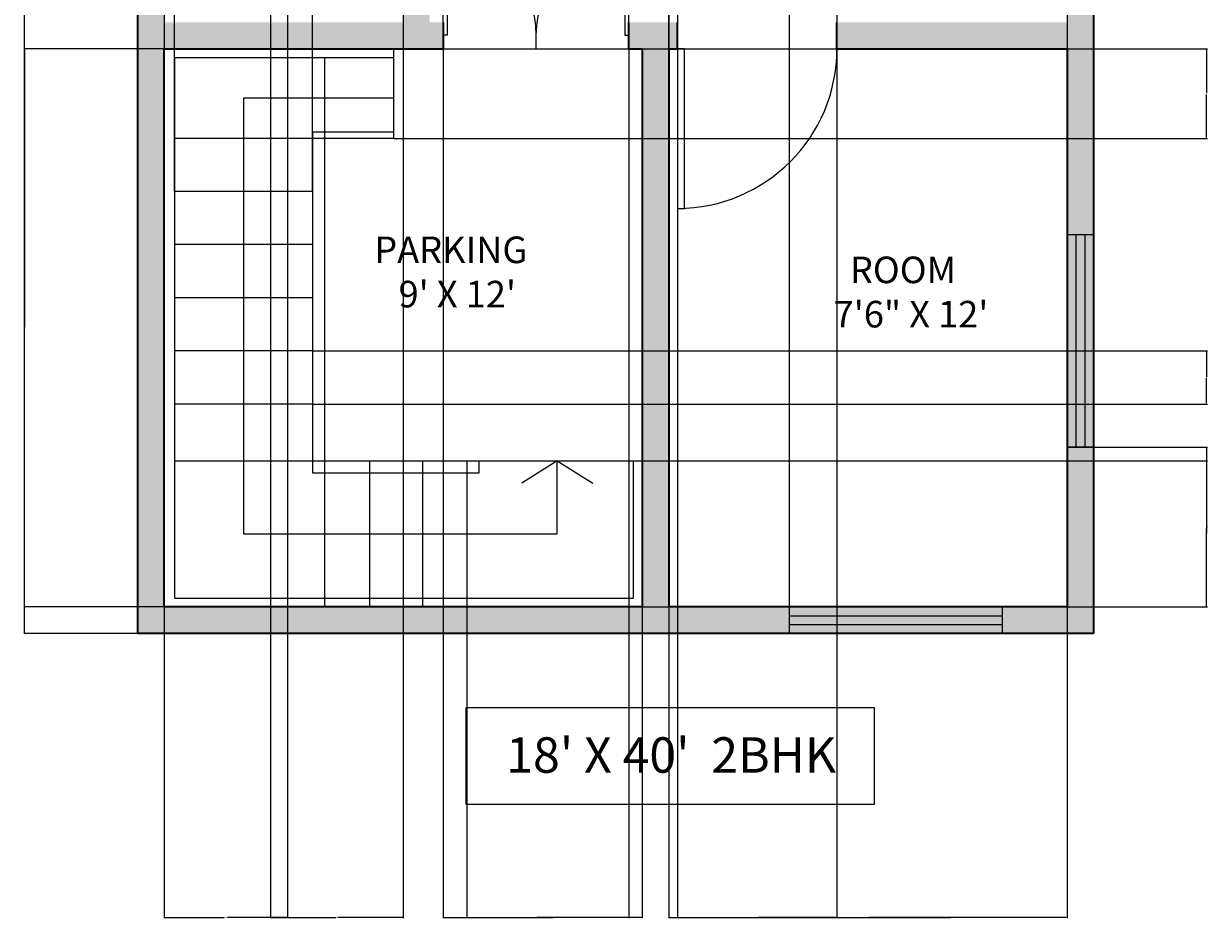
# Model space of a CAD drawing. Units: feet. Extents: x 4596233 to 4596501, y 5666486 to 5667044.
# Tile 1 of 3: x 4596233 to 4596501, y 5666486 to 5666688. Entities that reach past the tile are written whole.
import ezdxf

# ---------------------------------------------------------------- set-up
doc = ezdxf.new("R2010")
doc.units = ezdxf.units.FT
for name, color, linetype, lineweight in [('A-ANNO-DIMS', 2, 'Continuous', 18), ('A-ANNO-TTLB', 6, 'Continuous', 25), ('A-WALL', 7, 'Continuous', 35), ('ANNOTATION', 170, 'Continuous', 18), ('DOOR', 240, 'Continuous', 18), ('STAIR', 90, 'Continuous', 25)]:
    doc.layers.add(name, color=color, linetype=linetype, lineweight=lineweight)
doc.layers.add('A-GLAZ', color=2, linetype='Continuous', lineweight=18, true_color=0xf1eb1f)
doc.layers.add('A-WALL-PATT', color=251, linetype='Continuous', lineweight=13, true_color=0x636466)
doc.styles.get("Standard").update_dxf_attribs({"font": 'arial.ttf'})
doc.dimstyles.get("Standard").update_dxf_attribs({"dimtxt": 0.18, "dimasz": 0.18, "dimexe": 0.18, "dimexo": 0.0625, "dimgap": 0.09, "dimtad": 0, "dimtih": 1, "dimtoh": 1, "dimdec": 0, "dimzin": 0, "dimdsep": 46, "dimlunit": 3, "dimtxsty": 'Standard', "dimcen": 0.09, "dimadec": 0, "dimazin": 0, "dimtfac": 1, "dimtdec": 0, "dimtofl": 0, "dimtmove": 0, "dimatfit": 3, "dimfxl": 1, "dimtolj": 1, "dimtzin": 0, "dimarcsym": 0})

# ---------------------------------------------------------------- blocks, each defined once
blk = doc.blocks.new('*U3')
for p, q in [((0, 0), (0, -6)), ((-40, 0), (-40, -6))]:
    blk.add_line(p, q)
blk.add_lwpolyline([(0, 0), (0, 40), (-1.75, 40), (-1.75, 0)], close=True)
blk.add_arc((0, 0), 40, 90, 180)
blk = doc.blocks.new('*U4')
for p, q in [((0, 0), (0, 6)), ((40, 0), (40, 6))]:
    blk.add_line(p, q)
blk.add_lwpolyline([(0, 0), (0, -40), (1.75, -40), (1.75, 0)], close=True)
blk.add_arc((0, 0), 40, 270, 0)
blk = doc.blocks.new('WIN-48IN')
h = blk.add_hatch(color=256)
h.dxf.hatch_style = 1
h.paths.add_polyline_path([(48, 2), (48, 4), (0, 4), (0, 2)])
for p, q in [((0, 6), (48, 6)), ((0, 0), (0, 6)), ((48, 6), (48, 0)), ((0, 4), (48, 4)), ((0, 2), (48, 2)), ((48, 0), (0, 0))]:
    blk.add_line(p, q)
blk = doc.blocks.new('*D12')
at = {"layer": 'A-ANNO-DIMS', "color": 0, "lineweight": -2, "transparency": 16777216}
for p, q in [((4596258.79, 5667018.15), (4596233.12, 5667018.15)), ((4596233.3, 5667017.97), (4596233.3, 5666784.33)), ((4596233.3, 5666550.33), (4596233.3, 5666783.97)), ((4596258.79, 5666550.15), (4596233.12, 5666550.15))]:
    blk.add_line(p, q, dxfattribs=at)
at = {"layer": 'A-ANNO-DIMS', "color": 0, "transparency": 16777216}
for points in [[(4596233.27, 5667017.97), (4596233.33, 5667017.97), (4596233.3, 5667018.15)], [(4596233.27, 5666550.33), (4596233.33, 5666550.33), (4596233.3, 5666550.15)]]:
    blk.add_solid(points, dxfattribs=at)
at = {"layer": 'Defpoints', "color": 0, "transparency": 16777216}
for p in [(4596233.3, 5667018.15), (4596258.85, 5667018.15), (4596258.85, 5666550.15)]:
    blk.add_point(p, dxfattribs=at)
at = {"layer": 'A-ANNO-DIMS', "color": 0, "transparency": 16777216, "insert": (4596233.3, 5666784.15), "char_height": 0.18, "attachment_point": 5}
blk.add_mtext('\\A1;468', dxfattribs=at)
blk = doc.blocks.new('*D13')
at = {"layer": 'A-ANNO-DIMS', "color": 0, "lineweight": -2, "transparency": 16777216}
for p, q in [((4596264.79, 5666682.15), (4596233.12, 5666682.15)), ((4596233.3, 5666681.97), (4596233.3, 5666619.33)), ((4596233.3, 5666556.33), (4596233.3, 5666618.97)), ((4596264.79, 5666556.15), (4596233.12, 5666556.15))]:
    blk.add_line(p, q, dxfattribs=at)
at = {"layer": 'A-ANNO-DIMS', "color": 0, "transparency": 16777216}
for points in [[(4596233.27, 5666681.97), (4596233.33, 5666681.97), (4596233.3, 5666682.15)], [(4596233.27, 5666556.33), (4596233.33, 5666556.33), (4596233.3, 5666556.15)]]:
    blk.add_solid(points, dxfattribs=at)
at = {"layer": 'Defpoints', "color": 0, "transparency": 16777216}
for p in [(4596233.3, 5666682.15), (4596264.85, 5666682.15), (4596264.85, 5666556.15)]:
    blk.add_point(p, dxfattribs=at)
at = {"layer": 'A-ANNO-DIMS', "color": 0, "transparency": 16777216, "insert": (4596233.3, 5666619.15), "char_height": 0.18, "attachment_point": 5}
blk.add_mtext('\\A1;126', dxfattribs=at)
blk = doc.blocks.new('*D15')
at = {"layer": 'A-ANNO-DIMS', "color": 0, "lineweight": -2, "transparency": 16777216}
for p, q in [((4596378.85, 5666964.09), (4596378.85, 5666485.84)), ((4596468.85, 5666964.09), (4596468.85, 5666485.84)), ((4596379.03, 5666486.02), (4596423.63, 5666486.02)), ((4596468.67, 5666486.02), (4596424.07, 5666486.02))]:
    blk.add_line(p, q, dxfattribs=at)
at = {"layer": 'A-ANNO-DIMS', "color": 0, "transparency": 16777216}
for points in [[(4596379.03, 5666486.05), (4596379.03, 5666485.99), (4596378.85, 5666486.02)], [(4596468.67, 5666486.05), (4596468.67, 5666485.99), (4596468.85, 5666486.02)]]:
    blk.add_solid(points, dxfattribs=at)
at = {"layer": 'Defpoints', "color": 0, "transparency": 16777216}
for p in [(4596378.85, 5666964.15), (4596468.85, 5666964.15), (4596468.85, 5666486.02)]:
    blk.add_point(p, dxfattribs=at)
at = {"layer": 'A-ANNO-DIMS', "color": 0, "transparency": 16777216, "insert": (4596423.85, 5666486.02), "char_height": 0.18, "attachment_point": 5}
blk.add_mtext('\\A1;90', dxfattribs=at)
blk = doc.blocks.new('*D16')
at = {"layer": 'A-ANNO-DIMS', "color": 0, "lineweight": -2, "transparency": 16777216}
for p, q in [((4596327.85, 5666682.09), (4596327.85, 5666485.84)), ((4596369.85, 5666682.09), (4596369.85, 5666485.84)), ((4596328.03, 5666486.02), (4596348.63, 5666486.02)), ((4596369.67, 5666486.02), (4596349.07, 5666486.02))]:
    blk.add_line(p, q, dxfattribs=at)
at = {"layer": 'A-ANNO-DIMS', "color": 0, "transparency": 16777216}
for points in [[(4596328.03, 5666486.05), (4596328.03, 5666485.99), (4596327.85, 5666486.02)], [(4596369.67, 5666486.05), (4596369.67, 5666485.99), (4596369.85, 5666486.02)]]:
    blk.add_solid(points, dxfattribs=at)
at = {"layer": 'Defpoints', "color": 0, "transparency": 16777216}
for p in [(4596327.85, 5666682.15), (4596369.85, 5666682.15), (4596369.85, 5666486.02)]:
    blk.add_point(p, dxfattribs=at)
at = {"layer": 'A-ANNO-DIMS', "color": 0, "transparency": 16777216, "insert": (4596348.85, 5666486.02), "char_height": 0.18, "attachment_point": 5}
blk.add_mtext('\\A1;42', dxfattribs=at)
blk = doc.blocks.new('*D18')
at = {"layer": 'A-ANNO-DIMS', "color": 0, "lineweight": -2, "transparency": 16777216}
for p, q in [((4596288.85, 5666814.09), (4596288.85, 5666485.84)), ((4596318.85, 5666814.09), (4596318.85, 5666485.84)), ((4596289.03, 5666486.02), (4596303.63, 5666486.02)), ((4596318.67, 5666486.02), (4596304.07, 5666486.02))]:
    blk.add_line(p, q, dxfattribs=at)
at = {"layer": 'A-ANNO-DIMS', "color": 0, "transparency": 16777216}
for points in [[(4596289.03, 5666486.05), (4596289.03, 5666485.99), (4596288.85, 5666486.02)], [(4596318.67, 5666486.05), (4596318.67, 5666485.99), (4596318.85, 5666486.02)]]:
    blk.add_solid(points, dxfattribs=at)
at = {"layer": 'Defpoints', "color": 0, "transparency": 16777216}
for p in [(4596288.85, 5666814.15), (4596318.85, 5666814.15), (4596318.85, 5666486.02)]:
    blk.add_point(p, dxfattribs=at)
at = {"layer": 'A-ANNO-DIMS', "color": 0, "transparency": 16777216, "insert": (4596303.85, 5666486.02), "char_height": 0.18, "attachment_point": 5}
blk.add_mtext('\\A1;30', dxfattribs=at)
blk = doc.blocks.new('*D21')
at = {"layer": 'A-ANNO-DIMS', "color": 0, "lineweight": -2, "transparency": 16777216}
for p, q in [((4596380.85, 5666886.09), (4596380.85, 5666485.84)), ((4596416.85, 5666886.09), (4596416.85, 5666485.84)), ((4596381.03, 5666486.02), (4596398.63, 5666486.02)), ((4596416.67, 5666486.02), (4596399.07, 5666486.02))]:
    blk.add_line(p, q, dxfattribs=at)
at = {"layer": 'A-ANNO-DIMS', "color": 0, "transparency": 16777216}
for points in [[(4596381.03, 5666486.05), (4596381.03, 5666485.99), (4596380.85, 5666486.02)], [(4596416.67, 5666486.05), (4596416.67, 5666485.99), (4596416.85, 5666486.02)]]:
    blk.add_solid(points, dxfattribs=at)
at = {"layer": 'Defpoints', "color": 0, "transparency": 16777216}
for p in [(4596380.85, 5666886.15), (4596416.85, 5666886.15), (4596416.85, 5666486.02)]:
    blk.add_point(p, dxfattribs=at)
at = {"layer": 'A-ANNO-DIMS', "color": 0, "transparency": 16777216, "insert": (4596398.85, 5666486.02), "char_height": 0.18, "attachment_point": 5}
blk.add_mtext('\\A1;36', dxfattribs=at)
blk = doc.blocks.new('*D22')
at = {"layer": 'A-ANNO-DIMS', "color": 0, "lineweight": -2, "transparency": 16777216}
for p, q in [((4596264.85, 5667012.09), (4596264.85, 5666485.84)), ((4596292.72, 5667012.09), (4596292.72, 5666485.84)), ((4596265.03, 5666486.02), (4596278.39, 5666486.02)), ((4596292.54, 5666486.02), (4596279.18, 5666486.02))]:
    blk.add_line(p, q, dxfattribs=at)
at = {"layer": 'A-ANNO-DIMS', "color": 0, "transparency": 16777216}
for points in [[(4596265.03, 5666486.05), (4596265.03, 5666485.99), (4596264.85, 5666486.02)], [(4596292.54, 5666486.05), (4596292.54, 5666485.99), (4596292.72, 5666486.02)]]:
    blk.add_solid(points, dxfattribs=at)
at = {"layer": 'Defpoints', "color": 0, "transparency": 16777216}
for p in [(4596264.85, 5667012.15), (4596292.72, 5667012.15), (4596292.72, 5666486.02)]:
    blk.add_point(p, dxfattribs=at)
at = {"layer": 'A-ANNO-DIMS', "color": 0, "transparency": 16777216, "insert": (4596278.78, 5666486.02), "char_height": 0.18, "attachment_point": 5}
blk.add_mtext('\\A1;27.87', dxfattribs=at)
blk = doc.blocks.new('*D27')
at = {"layer": 'A-ANNO-DIMS', "color": 0, "lineweight": -2, "transparency": 16777216}
for p, q in [((4596468.91, 5666592.24), (4596500.58, 5666592.24)), ((4596500.4, 5666592.06), (4596500.4, 5666574.38)), ((4596500.4, 5666556.33), (4596500.4, 5666574.01)), ((4596468.91, 5666556.15), (4596500.58, 5666556.15))]:
    blk.add_line(p, q, dxfattribs=at)
at = {"layer": 'A-ANNO-DIMS', "color": 0, "transparency": 16777216}
for points in [[(4596500.37, 5666592.06), (4596500.43, 5666592.06), (4596500.4, 5666592.24)], [(4596500.37, 5666556.33), (4596500.43, 5666556.33), (4596500.4, 5666556.15)]]:
    blk.add_solid(points, dxfattribs=at)
at = {"layer": 'Defpoints', "color": 0, "transparency": 16777216}
for p in [(4596468.85, 5666592.24), (4596500.4, 5666592.24), (4596468.85, 5666556.15)]:
    blk.add_point(p, dxfattribs=at)
at = {"layer": 'A-ANNO-DIMS', "color": 0, "transparency": 16777216, "insert": (4596500.4, 5666574.19), "char_height": 0.18, "attachment_point": 5}
blk.add_mtext('\\A1;36.09', dxfattribs=at)
blk = doc.blocks.new('*D28')
at = {"layer": 'A-ANNO-DIMS', "color": 0, "lineweight": -2, "transparency": 16777216}
for p, q in [((4596378.85, 5666556.21), (4596378.85, 5667043.88)), ((4596379.03, 5667043.7), (4596392.04, 5667043.7)), ((4596405.99, 5667043.7), (4596392.97, 5667043.7)), ((4596406.17, 5666556.21), (4596406.17, 5667043.88))]:
    blk.add_line(p, q, dxfattribs=at)
at = {"layer": 'A-ANNO-DIMS', "color": 0, "transparency": 16777216}
for points in [[(4596379.03, 5667043.73), (4596379.03, 5667043.67), (4596378.85, 5667043.7)], [(4596405.99, 5667043.73), (4596405.99, 5667043.67), (4596406.17, 5667043.7)]]:
    blk.add_solid(points, dxfattribs=at)
at = {"layer": 'Defpoints', "color": 0, "transparency": 16777216}
for p in [(4596406.17, 5667043.7), (4596378.85, 5666556.15), (4596406.17, 5666556.15)]:
    blk.add_point(p, dxfattribs=at)
at = {"layer": 'A-ANNO-DIMS', "color": 0, "transparency": 16777216, "insert": (4596392.51, 5667043.7), "char_height": 0.18, "attachment_point": 5}
blk.add_mtext('\\A1;27.317', dxfattribs=at)
blk = doc.blocks.new('*D32')
at = {"layer": 'A-ANNO-DIMS', "color": 0, "lineweight": -2, "transparency": 16777216}
for p, q in [((4596298.41, 5666613.96), (4596500.58, 5666613.96)), ((4596500.4, 5666613.78), (4596500.4, 5666608.14)), ((4596500.4, 5666602.14), (4596500.4, 5666607.78)), ((4596298.41, 5666601.96), (4596500.58, 5666601.96))]:
    blk.add_line(p, q, dxfattribs=at)
at = {"layer": 'A-ANNO-DIMS', "color": 0, "transparency": 16777216}
for points in [[(4596500.37, 5666613.78), (4596500.43, 5666613.78), (4596500.4, 5666613.96)], [(4596500.37, 5666602.14), (4596500.43, 5666602.14), (4596500.4, 5666601.96)]]:
    blk.add_solid(points, dxfattribs=at)
at = {"layer": 'Defpoints', "color": 0, "transparency": 16777216}
for p in [(4596298.35, 5666613.96), (4596500.4, 5666613.96), (4596298.35, 5666601.96)]:
    blk.add_point(p, dxfattribs=at)
at = {"layer": 'A-ANNO-DIMS', "color": 0, "transparency": 16777216, "insert": (4596500.4, 5666607.96), "char_height": 0.18, "attachment_point": 5}
blk.add_mtext('\\A1;12', dxfattribs=at)
blk = doc.blocks.new('*D33')
at = {"layer": 'A-ANNO-DIMS', "color": 0, "lineweight": -2, "transparency": 16777216}
for p, q in [((4596267.15, 5666650.02), (4596267.15, 5667043.88)), ((4596267.33, 5667043.7), (4596282.36, 5667043.7)), ((4596298.17, 5667043.7), (4596283.14, 5667043.7)), ((4596298.35, 5666650.02), (4596298.35, 5667043.88))]:
    blk.add_line(p, q, dxfattribs=at)
at = {"layer": 'A-ANNO-DIMS', "color": 0, "transparency": 16777216}
for points in [[(4596267.33, 5667043.73), (4596267.33, 5667043.67), (4596267.15, 5667043.7)], [(4596298.17, 5667043.73), (4596298.17, 5667043.67), (4596298.35, 5667043.7)]]:
    blk.add_solid(points, dxfattribs=at)
at = {"layer": 'Defpoints', "color": 0, "transparency": 16777216}
for p in [(4596298.35, 5667043.7), (4596267.15, 5666649.96), (4596298.35, 5666649.96)]:
    blk.add_point(p, dxfattribs=at)
at = {"layer": 'A-ANNO-DIMS', "color": 0, "transparency": 16777216, "insert": (4596282.75, 5667043.7), "char_height": 0.18, "attachment_point": 5}
blk.add_mtext('\\A1;31.19', dxfattribs=at)
blk = doc.blocks.new('*D38')
at = {"layer": 'A-ANNO-DIMS', "color": 0, "lineweight": -2, "transparency": 16777216}
for p, q in [((4596416.85, 5666886.09), (4596416.85, 5666485.84)), ((4596468.85, 5666886.09), (4596468.85, 5666485.84)), ((4596417.03, 5666486.02), (4596442.63, 5666486.02)), ((4596468.67, 5666486.02), (4596443.07, 5666486.02))]:
    blk.add_line(p, q, dxfattribs=at)
at = {"layer": 'A-ANNO-DIMS', "color": 0, "transparency": 16777216}
for points in [[(4596417.03, 5666486.05), (4596417.03, 5666485.99), (4596416.85, 5666486.02)], [(4596468.67, 5666486.05), (4596468.67, 5666485.99), (4596468.85, 5666486.02)]]:
    blk.add_solid(points, dxfattribs=at)
at = {"layer": 'Defpoints', "color": 0, "transparency": 16777216}
for p in [(4596416.85, 5666886.15), (4596468.85, 5666886.15), (4596468.85, 5666486.02)]:
    blk.add_point(p, dxfattribs=at)
at = {"layer": 'A-ANNO-DIMS', "color": 0, "transparency": 16777216, "insert": (4596442.85, 5666486.02), "char_height": 0.18, "attachment_point": 5}
blk.add_mtext('\\A1;52', dxfattribs=at)
blk = doc.blocks.new('*D40')
at = {"layer": 'A-ANNO-DIMS', "color": 0, "lineweight": -2, "transparency": 16777216}
for p, q in [((4596333.21, 5666556.09), (4596333.21, 5666485.84)), ((4596372.85, 5666556.09), (4596372.85, 5666485.84)), ((4596333.39, 5666486.02), (4596352.64, 5666486.02)), ((4596372.67, 5666486.02), (4596353.42, 5666486.02))]:
    blk.add_line(p, q, dxfattribs=at)
at = {"layer": 'A-ANNO-DIMS', "color": 0, "transparency": 16777216}
for points in [[(4596333.39, 5666486.05), (4596333.39, 5666485.99), (4596333.21, 5666486.02)], [(4596372.67, 5666486.05), (4596372.67, 5666485.99), (4596372.85, 5666486.02)]]:
    blk.add_solid(points, dxfattribs=at)
at = {"layer": 'Defpoints', "color": 0, "transparency": 16777216}
for p in [(4596333.21, 5666556.15), (4596372.85, 5666556.15), (4596372.85, 5666486.02)]:
    blk.add_point(p, dxfattribs=at)
at = {"layer": 'A-ANNO-DIMS', "color": 0, "transparency": 16777216, "insert": (4596353.03, 5666486.02), "char_height": 0.18, "attachment_point": 5}
blk.add_mtext('\\A1;39.64', dxfattribs=at)
blk = doc.blocks.new('*D41')
at = {"layer": 'A-ANNO-DIMS', "color": 0, "lineweight": -2, "transparency": 16777216}
for p, q in [((4596372.91, 5666589.12), (4596500.58, 5666589.12)), ((4596500.4, 5666588.94), (4596500.4, 5666572.82)), ((4596500.4, 5666556.33), (4596500.4, 5666572.45)), ((4596372.91, 5666556.15), (4596500.58, 5666556.15))]:
    blk.add_line(p, q, dxfattribs=at)
at = {"layer": 'A-ANNO-DIMS', "color": 0, "transparency": 16777216}
for points in [[(4596500.37, 5666588.94), (4596500.43, 5666588.94), (4596500.4, 5666589.12)], [(4596500.37, 5666556.33), (4596500.43, 5666556.33), (4596500.4, 5666556.15)]]:
    blk.add_solid(points, dxfattribs=at)
at = {"layer": 'Defpoints', "color": 0, "transparency": 16777216}
for p in [(4596372.85, 5666589.12), (4596500.4, 5666589.12), (4596372.85, 5666556.15)]:
    blk.add_point(p, dxfattribs=at)
at = {"layer": 'A-ANNO-DIMS', "color": 0, "transparency": 16777216, "insert": (4596500.4, 5666572.63), "char_height": 0.18, "attachment_point": 5}
blk.add_mtext('\\A1;32.97', dxfattribs=at)
blk = doc.blocks.new('*D42')
at = {"layer": 'A-ANNO-DIMS', "color": 0, "lineweight": -2, "transparency": 16777216}
for p, q in [((4596316.7, 5666682.15), (4596500.58, 5666682.15)), ((4596500.4, 5666681.97), (4596500.4, 5666672.24)), ((4596500.4, 5666662.14), (4596500.4, 5666671.87)), ((4596316.7, 5666661.96), (4596500.58, 5666661.96))]:
    blk.add_line(p, q, dxfattribs=at)
at = {"layer": 'A-ANNO-DIMS', "color": 0, "transparency": 16777216}
for points in [[(4596500.37, 5666681.97), (4596500.43, 5666681.97), (4596500.4, 5666682.15)], [(4596500.37, 5666662.14), (4596500.43, 5666662.14), (4596500.4, 5666661.96)]]:
    blk.add_solid(points, dxfattribs=at)
at = {"layer": 'Defpoints', "color": 0, "transparency": 16777216}
for p in [(4596316.63, 5666682.15), (4596500.4, 5666682.15), (4596316.63, 5666661.96)]:
    blk.add_point(p, dxfattribs=at)
at = {"layer": 'A-ANNO-DIMS', "color": 0, "transparency": 16777216, "insert": (4596500.4, 5666672.05), "char_height": 0.18, "attachment_point": 5}
blk.add_mtext('\\A1;20.187', dxfattribs=at)

msp = doc.modelspace()

# ---------------------------------------------------------------- hatches: boundary and pattern name
at = {"layer": 'A-WALL-PATT'}
h = msp.add_hatch(color=256, dxfattribs=at)
h.dxf.hatch_style = 1
h.paths.add_polyline_path([(4596474.8511, 5667018.1479), (4596258.8511, 5667018.1479), (4596258.8511, 5666550.1479), (4596474.8511, 5666550.1479)])
h.paths.add_polyline_path([(4596372.8511, 5667012.1479), (4596372.8511, 5666892.1479), (4596370.8511, 5666892.1479), (4596370.8511, 5666891.5479), (4596370.8511, 5666886.1479), (4596380.8511, 5666886.1479), (4596380.8511, 5666892.1479), (4596378.8511, 5666892.1479), (4596378.8511, 5666964.1479), (4596380.8511, 5666964.1479), (4596380.8511, 5666970.1479), (4596378.8511, 5666970.1479), (4596378.8511, 5667012.1479), (4596468.8511, 5667012.1479), (4596468.8511, 5666970.1479), (4596416.8511, 5666970.1479), (4596416.8511, 5666964.1479), (4596468.8511, 5666964.1479), (4596468.8511, 5666892.1479), (4596416.8511, 5666892.1479), (4596416.8511, 5666886.1479), (4596468.8511, 5666886.1479), (4596468.8511, 5666688.1479), (4596416.8511, 5666688.1479), (4596416.8511, 5666682.1479), (4596468.8511, 5666682.1479), (4596468.8511, 5666556.1479), (4596378.8511, 5666556.1479), (4596378.8511, 5666682.1479), (4596380.8511, 5666682.1479), (4596380.8511, 5666687.5479), (4596380.8511, 5666688.1479), (4596369.8511, 5666688.1479), (4596369.8511, 5666685.2979), (4596369.8511, 5666682.1479), (4596372.8511, 5666682.1479), (4596372.8511, 5666556.1479), (4596264.8511, 5666556.1479), (4596264.8511, 5666682.1479), (4596327.8511, 5666682.1479), (4596327.8511, 5666685.2979), (4596327.8511, 5666688.1479), (4596324.8511, 5666688.1479), (4596324.8511, 5666772.1479), (4596318.8511, 5666772.1479), (4596318.8511, 5666760.1479), (4596318.8511, 5666754.1479), (4596318.8511, 5666724.1479), (4596318.8511, 5666688.1479), (4596264.8511, 5666688.1479), (4596264.8511, 5666754.1479), (4596288.8511, 5666754.1479), (4596288.8511, 5666758.6479), (4596288.8511, 5666760.1479), (4596264.8511, 5666760.1479), (4596264.8511, 5666814.1479), (4596288.8511, 5666814.1479), (4596288.8511, 5666818.6479), (4596288.8511, 5666820.1479), (4596264.8511, 5666820.1479), (4596264.8511, 5666886.1479), (4596318.8511, 5666886.1479), (4596318.8511, 5666820.1479), (4596318.8511, 5666818.6479), (4596318.8511, 5666814.1479), (4596318.8511, 5666802.1479), (4596324.8511, 5666802.1479), (4596324.8511, 5666886.1479), (4596334.8511, 5666886.1479), (4596334.8511, 5666891.5479), (4596334.8511, 5666892.1479), (4596264.8511, 5666892.1479), (4596264.8511, 5667012.1479)], flags=16)
h.paths.add_polyline_path([(4596316.6338, 5666680.1479), (4596316.6338, 5666661.9608), (4596301.036, 5666661.9608), (4596301.036, 5666589.119), (4596370.916, 5666589.119), (4596370.916, 5666558.119), (4596267.1547, 5666558.119), (4596267.1547, 5666680.1479)], flags=0)
h.paths.add_polyline_path([(4596282.7503, 5666649.9608), (4596298.3459, 5666649.9608), (4596298.3459, 5666586.4128), (4596333.2108, 5666586.4128), (4596333.2108, 5666572.6335), (4596282.7503, 5666572.6335)], flags=0)
h.paths.add_polyline_path([(4596380.8511, 5666682.1479), (4596382.4261, 5666682.1479), (4596382.4261, 5666646.1479), (4596380.8511, 5666646.1479)], flags=0)
h.paths.add_polyline_path([(4596270.4341, 5666856.9819), (4596311.4805, 5666856.9819), (4596311.4805, 5666879.3708), (4596270.4341, 5666879.3708)], flags=8)
h.paths.add_polyline_path([(4596271.3283, 5666778.1649), (4596312.3747, 5666778.1649), (4596312.3747, 5666800.5538), (4596271.3283, 5666800.5538)], flags=8)
h.paths.add_polyline_path([(4596401.0723, 5666924.3036), (4596440.8622, 5666924.3036), (4596440.8622, 5666946.6925), (4596401.0723, 5666946.6925)], flags=8)
h.paths.add_polyline_path([(4596396.1839, 5666976.1395), (4596449.4963, 5666976.1395), (4596449.4963, 5666998.5283), (4596396.1839, 5666998.5283)], flags=8)
h.paths.add_polyline_path([(4596288.0879, 5666956.0844), (4596336.7264, 5666956.0844), (4596336.7264, 5666978.4732), (4596288.0879, 5666978.4732)], flags=8)
h.paths.add_polyline_path([(4596267.7433, 5666702.4027), (4596308.7897, 5666702.4027), (4596308.7897, 5666724.7916), (4596267.7433, 5666724.7916)], flags=8)
h.paths.add_polyline_path([(4596371.4978, 5666770.3665), (4596425.2768, 5666770.3665), (4596425.2768, 5666792.7553), (4596371.4978, 5666792.7553)], flags=8)
h.paths.add_polyline_path([(4596414.2198, 5666615.8536), (4596452.2908, 5666615.8536), (4596452.2908, 5666638.2424), (4596414.2198, 5666638.2424)], flags=8)
h.paths.add_polyline_path([(4596310.1554, 5666620.3865), (4596350.8825, 5666620.3865), (4596350.8825, 5666642.7753), (4596310.1554, 5666642.7753)], flags=8)
h = msp.add_hatch(color=256, dxfattribs=at)
h.dxf.hatch_style = 1
h.paths.add_polyline_path([(4596474.8511, 5667018.1479), (4596258.8511, 5667018.1479), (4596258.8511, 5666550.1479), (4596474.8511, 5666550.1479)])
h.paths.add_polyline_path([(4596468.8511, 5666970.1479), (4596416.8511, 5666970.1479), (4596416.8511, 5666964.1479), (4596468.8511, 5666964.1479), (4596468.8511, 5666892.1479), (4596416.8511, 5666892.1479), (4596416.8511, 5666886.1479), (4596468.8511, 5666886.1479), (4596468.8511, 5666688.1479), (4596416.8511, 5666688.1479), (4596416.8511, 5666682.1479), (4596468.8511, 5666682.1479), (4596468.8511, 5666556.1479), (4596378.8511, 5666556.1479), (4596378.8511, 5666682.1479), (4596380.8511, 5666682.1479), (4596380.8511, 5666687.5479), (4596380.8511, 5666688.1479), (4596369.8511, 5666688.1479), (4596369.8511, 5666685.2979), (4596369.8511, 5666682.1479), (4596372.8511, 5666682.1479), (4596372.8511, 5666556.1479), (4596264.8511, 5666556.1479), (4596264.8511, 5666682.1479), (4596327.8511, 5666682.1479), (4596327.8511, 5666685.2979), (4596327.8511, 5666688.1479), (4596324.8511, 5666688.1479), (4596324.8511, 5666772.1479), (4596318.8511, 5666772.1479), (4596318.8511, 5666760.1479), (4596318.8511, 5666754.1479), (4596318.8511, 5666724.1479), (4596318.8511, 5666688.1479), (4596264.8511, 5666688.1479), (4596264.8511, 5666754.1479), (4596288.8511, 5666754.1479), (4596288.8511, 5666758.6479), (4596288.8511, 5666760.1479), (4596264.8511, 5666760.1479), (4596264.8511, 5666814.1479), (4596288.8511, 5666814.1479), (4596288.8511, 5666818.6479), (4596288.8511, 5666820.1479), (4596264.8511, 5666820.1479), (4596264.8511, 5666886.1479), (4596318.8511, 5666886.1479), (4596318.8511, 5666820.1479), (4596318.8511, 5666818.6479), (4596318.8511, 5666814.1479), (4596318.8511, 5666802.1479), (4596324.8511, 5666802.1479), (4596324.8511, 5666886.1479), (4596334.8511, 5666886.1479), (4596334.8511, 5666891.5479), (4596334.8511, 5666892.1479), (4596264.8511, 5666892.1479), (4596264.8511, 5667012.1479), (4596372.8511, 5667012.1479), (4596372.8511, 5666892.1479), (4596370.8511, 5666892.1479), (4596370.8511, 5666891.5479), (4596370.8511, 5666886.1479), (4596380.8511, 5666886.1479), (4596380.8511, 5666892.1479), (4596378.8511, 5666892.1479), (4596378.8511, 5666964.1479), (4596380.8511, 5666964.1479), (4596380.8511, 5666970.1479), (4596378.8511, 5666970.1479), (4596378.8511, 5667012.1479), (4596468.8511, 5667012.1479)], flags=16)
h.paths.add_polyline_path([(4596382.4261, 5666646.1479), (4596380.8511, 5666646.1479), (4596380.8511, 5666682.1479), (4596382.4261, 5666682.1479)], flags=0)
h.paths.add_polyline_path([(4596316.6338, 5666680.1479), (4596316.6338, 5666661.9608), (4596301.036, 5666661.9608), (4596301.036, 5666589.119), (4596370.916, 5666589.119), (4596370.916, 5666558.119), (4596267.1547, 5666558.119), (4596267.1547, 5666680.1479)], flags=0)
h.paths.add_polyline_path([(4596282.7503, 5666649.9608), (4596298.3459, 5666649.9608), (4596298.3459, 5666586.4128), (4596333.2108, 5666586.4128), (4596333.2108, 5666572.6335), (4596282.7503, 5666572.6335)], flags=0)
h.paths.add_polyline_path([(4596270.4341, 5666856.9819), (4596311.4805, 5666856.9819), (4596311.4805, 5666879.3708), (4596270.4341, 5666879.3708)], flags=8)
h.paths.add_polyline_path([(4596271.3283, 5666778.1649), (4596312.3747, 5666778.1649), (4596312.3747, 5666800.5538), (4596271.3283, 5666800.5538)], flags=8)
h.paths.add_polyline_path([(4596401.0723, 5666924.3036), (4596440.8622, 5666924.3036), (4596440.8622, 5666946.6925), (4596401.0723, 5666946.6925)], flags=8)
h.paths.add_polyline_path([(4596396.1839, 5666976.1395), (4596449.4963, 5666976.1395), (4596449.4963, 5666998.5283), (4596396.1839, 5666998.5283)], flags=8)
h.paths.add_polyline_path([(4596288.0879, 5666956.0844), (4596336.7264, 5666956.0844), (4596336.7264, 5666978.4732), (4596288.0879, 5666978.4732)], flags=8)
h.paths.add_polyline_path([(4596267.7433, 5666702.4027), (4596308.7897, 5666702.4027), (4596308.7897, 5666724.7916), (4596267.7433, 5666724.7916)], flags=8)
h.paths.add_polyline_path([(4596371.4978, 5666770.3665), (4596425.2768, 5666770.3665), (4596425.2768, 5666792.7553), (4596371.4978, 5666792.7553)], flags=8)
h.paths.add_polyline_path([(4596414.2198, 5666615.8536), (4596452.2908, 5666615.8536), (4596452.2908, 5666638.2424), (4596414.2198, 5666638.2424)], flags=8)
h.paths.add_polyline_path([(4596310.1554, 5666620.3865), (4596350.8825, 5666620.3865), (4596350.8825, 5666642.7753), (4596310.1554, 5666642.7753)], flags=8)

# ---------------------------------------------------------------- linework, layer by layer
at = {"layer": 'A-ANNO-TTLB'}
msp.add_lwpolyline([(4596333.0933, 5666533.4276), (4596425.3012, 5666533.4276), (4596425.3012, 5666511.5729), (4596333.0933, 5666511.5729)], close=True, dxfattribs=at)
at = {"layer": 'A-WALL'}
for p, q in [((4596258.8511, 5666550.1479), (4596258.8511, 5667018.1479)), ((4596474.8511, 5667018.1479), (4596474.8511, 5666550.1479)), ((4596327.8511, 5666688.1479), (4596327.8511, 5666682.1479)), ((4596369.8511, 5666682.1479), (4596369.8511, 5666688.1479)), ((4596380.8511, 5666682.1479), (4596380.8511, 5666688.1479)), ((4596416.8511, 5666682.1479), (4596416.8511, 5666688.1479)), ((4596264.8511, 5666556.1479), (4596264.8511, 5666682.1479)), ((4596264.8511, 5666682.1479), (4596327.8511, 5666682.1479)), ((4596369.8511, 5666682.1479), (4596372.8511, 5666682.1479)), ((4596372.8511, 5666682.1479), (4596372.8511, 5666556.1479)), ((4596378.8511, 5666682.1479), (4596378.8511, 5666556.1479)), ((4596378.8511, 5666682.1479), (4596380.8511, 5666682.1479)), ((4596416.8511, 5666682.1479), (4596468.8511, 5666682.1479)), ((4596468.8511, 5666682.1479), (4596468.8511, 5666556.1479)), ((4596372.8511, 5666556.1479), (4596264.8511, 5666556.1479)), ((4596468.8511, 5666556.1479), (4596378.8511, 5666556.1479)), ((4596474.8511, 5666550.1479), (4596258.8511, 5666550.1479))]:
    msp.add_line(p, q, dxfattribs=at)
at = {"layer": 'STAIR'}
for p, q in [((4596316.6338, 5666680.1479), (4596267.1547, 5666680.1479)), ((4596267.1547, 5666680.1479), (4596267.1547, 5666558.119)), ((4596301.036, 5666680.1479), (4596301.036, 5666556.1479)), ((4596316.6338, 5666682.1479), (4596316.6338, 5666680.1479)), ((4596316.6338, 5666680.1479), (4596316.6338, 5666661.9608)), ((4596316.6338, 5666671.0544), (4596282.7503, 5666671.0544)), ((4596282.7503, 5666671.0544), (4596282.7503, 5666572.6335)), ((4596316.6338, 5666661.9608), (4596267.1547, 5666661.9608)), ((4596316.6338, 5666663.3592), (4596298.3459, 5666663.3592)), ((4596298.3459, 5666663.3592), (4596298.3459, 5666586.4128)), ((4596298.3459, 5666649.9608), (4596267.1547, 5666649.9608)), ((4596298.3459, 5666637.9608), (4596267.1547, 5666637.9608)), ((4596298.3459, 5666625.9608), (4596267.1547, 5666625.9608)), ((4596298.3459, 5666613.9608), (4596267.1547, 5666613.9608)), ((4596298.3459, 5666601.9608), (4596267.1547, 5666601.9608)), ((4596267.1547, 5666589.119), (4596370.916, 5666589.119)), ((4596311.2108, 5666589.119), (4596311.2108, 5666556.1479)), ((4596323.2108, 5666589.119), (4596323.2108, 5666556.1479)), ((4596333.2108, 5666589.119), (4596333.2108, 5666556.1479)), ((4596335.9997, 5666586.4128), (4596335.9997, 5666589.119)), ((4596353.678, 5666589.119), (4596345.6249, 5666584.0857)), ((4596353.678, 5666572.6335), (4596353.678, 5666589.119)), ((4596353.678, 5666589.119), (4596361.7311, 5666584.0857)), ((4596370.916, 5666558.119), (4596370.916, 5666589.119)), ((4596370.916, 5666589.119), (4596372.8511, 5666589.119)), ((4596298.3459, 5666586.4128), (4596335.9997, 5666586.4128)), ((4596282.7503, 5666572.6335), (4596353.678, 5666572.6335)), ((4596267.1547, 5666558.119), (4596370.916, 5666558.119))]:
    msp.add_line(p, q, dxfattribs=at)

# ---------------------------------------------------------------- block references
at = {"layer": 'A-GLAZ', "rotation": 270.000000006957}
msp.add_blockref('WIN-48IN', (4596468.8512, 5666640.2417), dxfattribs=at)
at = {"layer": 'A-GLAZ'}
msp.add_blockref('WIN-48IN', (4596406.1673, 5666550.148), dxfattribs=at)
at = {"layer": 'DOOR'}
for name, p, xscale, yscale, zscale in [('*U3', (4596327.8511, 5666685.2979), -0.5249999999945675, 0.5249999999945675, 0.5249999999945675), ('*U3', (4596369.8511, 5666685.2979), 0.5249999999945675, 0.5249999999945675, 0.5249999999945675), ('*U4', (4596380.8511, 5666682.1479), 0.8999999999906869, 0.8999999999906869, 0.8999999999906869)]:
    msp.add_blockref(name, p, dxfattribs=dict(at, xscale=xscale, yscale=yscale, zscale=zscale))

# ---------------------------------------------------------------- texts
at = {"layer": 'A-ANNO-TTLB', "insert": (4596342.1257, 5666526.7138), "char_height": 8, "attachment_point": 1}
msp.add_mtext_dynamic_manual_height_columns("18' X 40'  2BHK", width=87.464213, gutter_width=12.5, heights=[0], dxfattribs=at)
at = {"layer": 'ANNOTATION', "char_height": 6, "attachment_point": 1}
for s, width, insert in [("PARKING\\P   9' X 12'", 37.346852, (4596312.302, 5666639.7897)), ('  ROOM\\P7\'6" X 12\'', 37.807866, (4596416.1168, 5666635.2608))]:
    msp.add_mtext_dynamic_manual_height_columns(s, width=width, gutter_width=12.5, heights=[0], dxfattribs=dict(at, insert=insert))

# ---------------------------------------------------------------- dimensions: what is measured, and where the dimension line sits
at = {"layer": 'A-ANNO-DIMS'}
for base, p1, p2, override, picture, middle in [((4596298.3459, 5667043.6979), (4596267.1547, 5666649.9608), (4596298.3459, 5666649.9608), {"dimdec": 2, "dimlfac": 1, "dimrnd": 0, "dimzin": 0, "dimdsep": 46, "dimlunit": 2}, '*D33', (4596282.7503, 5667043.6979)), ((4596406.1677, 5667043.6979), (4596378.8511, 5666556.1479), (4596406.1677, 5666556.1479), {"dimdec": 3, "dimlfac": 1, "dimrnd": 0, "dimzin": 0, "dimdsep": 46, "dimlunit": 2}, '*D28', (4596392.5094, 5667043.6979)), ((4596292.7184, 5666486.0229), (4596264.8511, 5667012.1479), (4596292.7184, 5667012.1479), {"dimdec": 2, "dimlfac": 1, "dimrnd": 0, "dimzin": 0, "dimdsep": 46, "dimlunit": 2}, '*D22', (4596278.7847, 5666486.0229)), ((4596468.8511, 5666486.0229), (4596378.8511, 5666964.1479), (4596468.8511, 5666964.1479), {"dimdec": 0, "dimlfac": 1, "dimrnd": 0, "dimzin": 0, "dimdsep": 46, "dimlunit": 2}, '*D15', (4596423.8511, 5666486.0229)), ((4596416.8511, 5666486.0229), (4596380.8511, 5666886.1479), (4596416.8511, 5666886.1479), {"dimdec": 0, "dimlfac": 1, "dimrnd": 0, "dimzin": 0, "dimdsep": 46, "dimlunit": 2}, '*D21', (4596398.8511, 5666486.0229)), ((4596468.8511, 5666486.0229), (4596416.8511, 5666886.1479), (4596468.8511, 5666886.1479), {"dimdec": 0, "dimlfac": 1, "dimrnd": 0, "dimzin": 0, "dimdsep": 46, "dimlunit": 2}, '*D38', (4596442.8511, 5666486.0229)), ((4596318.8511, 5666486.0229), (4596288.8511, 5666814.1479), (4596318.8511, 5666814.1479), {"dimdec": 0, "dimlfac": 1, "dimrnd": 0, "dimzin": 0, "dimdsep": 46, "dimlunit": 2}, '*D18', (4596303.8511, 5666486.0229)), ((4596369.8511, 5666486.0229), (4596327.8511, 5666682.1479), (4596369.8511, 5666682.1479), {"dimdec": 0, "dimlfac": 1, "dimrnd": 0, "dimzin": 0, "dimdsep": 46, "dimlunit": 2}, '*D16', (4596348.8511, 5666486.0229)), ((4596372.8511, 5666486.0229), (4596333.2108, 5666556.1479), (4596372.8511, 5666556.1479), {"dimdec": 2, "dimlfac": 1, "dimrnd": 0, "dimzin": 0, "dimdsep": 46, "dimlunit": 2}, '*D40', (4596353.031, 5666486.0229))]:
    dim = msp.add_linear_dim(base=base, p1=p1, p2=p2, dimstyle='Standard', override=override, dxfattribs=at)
    dim.commit()
    dim.dimension.update_dxf_attribs({"geometry": picture, "text_midpoint": middle})
for base, p1, p2, override, picture, middle in [((4596233.3011, 5667018.1479), (4596258.8511, 5666550.1479), (4596258.8511, 5667018.1479), {"dimdec": 0, "dimlfac": 1, "dimrnd": 0, "dimzin": 0, "dimdsep": 46, "dimlunit": 2}, '*D12', (4596233.3011, 5666784.1479)), ((4596233.3011, 5666682.1479), (4596264.8511, 5666556.1479), (4596264.8511, 5666682.1479), {"dimdec": 0, "dimlfac": 1, "dimrnd": 0, "dimzin": 0, "dimdsep": 46, "dimlunit": 2}, '*D13', (4596233.3011, 5666619.1479)), ((4596500.4011, 5666682.1479), (4596316.6338, 5666661.9608), (4596316.6338, 5666682.1479), {"dimdec": 3, "dimlfac": 1, "dimrnd": 0, "dimzin": 0, "dimdsep": 46, "dimlunit": 2}, '*D42', (4596500.4011, 5666672.0544)), ((4596500.4011, 5666613.9608), (4596298.3459, 5666601.9608), (4596298.3459, 5666613.9608), {"dimdec": 0, "dimlfac": 1, "dimrnd": 0, "dimzin": 0, "dimdsep": 46, "dimlunit": 2}, '*D32', (4596500.4011, 5666607.9608)), ((4596500.4011, 5666592.2413), (4596468.8511, 5666556.1479), (4596468.8511, 5666592.2413), {"dimdec": 2, "dimlfac": 1, "dimrnd": 0, "dimzin": 0, "dimdsep": 46, "dimlunit": 2}, '*D27', (4596500.4011, 5666574.1946)), ((4596500.4011, 5666589.119), (4596372.8511, 5666556.1479), (4596372.8511, 5666589.119), {"dimdec": 2, "dimlfac": 1, "dimrnd": 0, "dimzin": 0, "dimdsep": 46, "dimlunit": 2}, '*D41', (4596500.4011, 5666572.6335))]:
    dim = msp.add_linear_dim(base=base, p1=p1, p2=p2, angle=90, dimstyle='Standard', override=override, dxfattribs=at)
    dim.commit()
    dim.dimension.update_dxf_attribs({"geometry": picture, "text_midpoint": middle})

doc.saveas('drawing.dxf')
